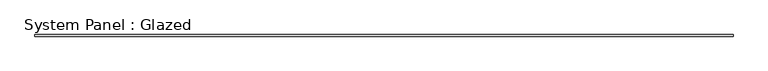
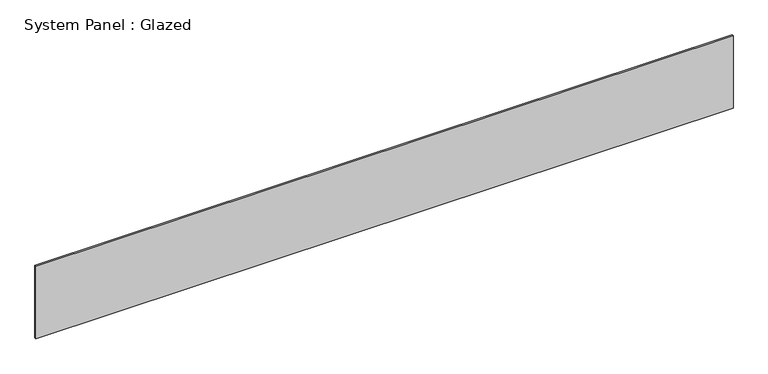
"""IFC4 building model written with IfcOpenShell, lengths in millimetres: plate geometry, System Panel : Glazed."""

from ifc_helpers import new_model, si_unit, origin, origin_with_axes, place, context, project, spatial, polyline, outline, extrude, source, transform, mapped, element, save


def system_panel_glazed_d9738348(model_context):
    return source(origin(), model_context, "Body", "SweptSolid", [
        extrude(outline(polyline([(5534.025, 19.05), (-5534.025, 19.05), (-5534.025, 44.45), (5534.025, 44.45), (5534.025, 19.05)])), origin_with_axes(), (0.0, 0.0, 1.0), 1219.2),
    ])


if __name__ == "__main__":
    model = new_model("IFC4")
    model_context = context("Model", 3, world=origin())
    ifc_project = project(units=[si_unit("LENGTHUNIT", "METRE", prefix="MILLI")], contexts=[model_context])
    site = spatial("IfcSite", under=ifc_project)
    building = spatial("IfcBuilding", under=site)
    placement = place(None, origin())
    system_panel_glazed_shape = system_panel_glazed_d9738348(model_context)
    element("IfcPlate", 1, ObjectType="System Panel : Glazed", at=placement, inside=building, context=model_context, shape_type="MappedRepresentation", body=[
        mapped(system_panel_glazed_shape, transform((0.0, 0.0, 0.0), x_axis=(1.0, 0.0, 0.0), y_axis=(0.0, 1.0, 0.0), z_axis=(0.0, 0.0, 1.0))),
    ])
    save(model, "model.ifc")

# Revit data of these elements
# Type "System Panel : Glazed"
#   Construction Type Id = "GSP4R"
#   Analytic Construction = "1/8 in Pilkington single glazing"
#   Visual Light Transmittance = 0.9
#   Solar Heat Gain Coefficient = 0.86
#   Heat Transfer Coefficient (U) = 1.18115 BTU/(h·ft²·°F)
# Element 1 (IfcPlate, "System Panel : Glazed")
#   Materials on its faces: "Glass"
# Materials
#   "Glass": class "Glass", colour RGB 0 128 192, transparency 0.75, Description = "Soda Lime Glass", Cost = 0
